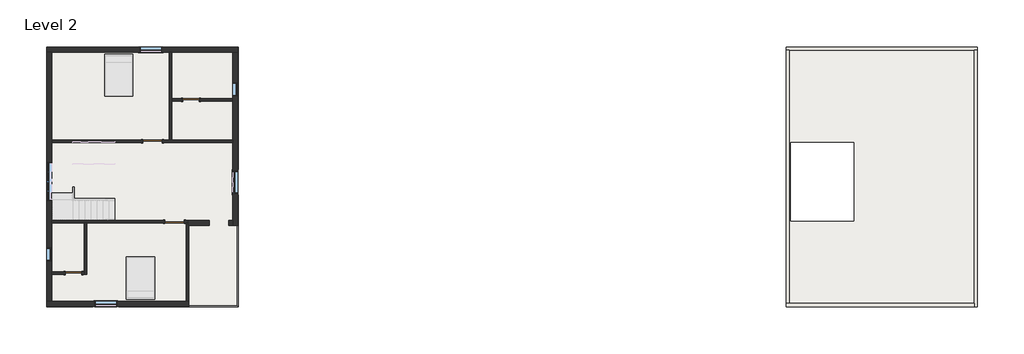
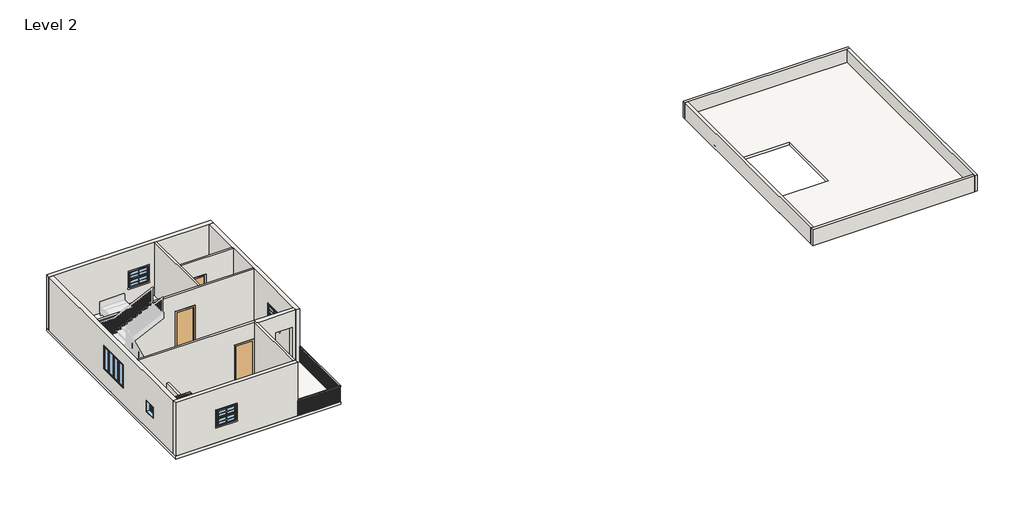
# One storey, part 1 of 3: 16 walls, 6 windows, 4 doors, 1 railing, 1 roof, 1 slab.
"""IFC4 building model written with IfcOpenShell, lengths in millimetres."""

from ifc_helpers import new_model, si_unit, frame, origin, place, context, project, spatial, polyline, outline, extrude, faceted_brep, transform, mapped, element, save
from components import door_f2b275c1, door_d8f5dbb5, single_flush_door_3_17d80c48, single_flush_door_3_5e62189b, window_fa0038f5, window_5487fb6d, window_f2d8fef0

model = new_model("IFC4")

# Units and contexts
model_context = context("Model", 3, world=origin())
ifc_project = project(units=[si_unit("LENGTHUNIT", "METRE", prefix="MILLI")], contexts=[model_context])

# Site, building, storey
site = spatial("IfcSite", under=ifc_project)
building = spatial("IfcBuilding", under=site)
storey = spatial("IfcBuildingStorey", under=building, Name="Level 2", Elevation=3048.0)

# Doors
placement = place(None, origin())
door_shape = door_f2b275c1(model_context)
element("IfcDoor", 1, ObjectType="Single-Flush : door 2'6\"", at=placement, inside=storey, context=model_context, shape_type="MappedRepresentation", body=[
    mapped(door_shape, transform((-16207.5289184, 4539.4100713, 3048.0), x_axis=(-1.0, 0.0, 0.0), y_axis=(0.0, -1.0, 0.0), z_axis=(0.0, 0.0, 1.0))),
])
door_2_shape = door_d8f5dbb5(model_context)
element("IfcDoor", 2, ObjectType="Single-Flush : door 2'6\"", at=placement, inside=storey, context=model_context, shape_type="MappedRepresentation", body=[
    mapped(door_2_shape, transform((-21693.9289184, -3575.8899287, 3048.0), x_axis=(1.0, 0.0, 0.0), y_axis=(0.0, 1.0, 0.0), z_axis=(0.0, 0.0, 1.0))),
])
single_flush_door_3_shape = single_flush_door_3_17d80c48(model_context)
element("IfcDoor", 3, ObjectType="Single-Flush : door 3'", at=placement, inside=storey, context=model_context, shape_type="MappedRepresentation", body=[
    mapped(single_flush_door_3_shape, transform((-18010.9289184, 2596.3100713, 3048.0), x_axis=(1.0, 0.0, 0.0), y_axis=(0.0, 1.0, 0.0), z_axis=(0.0, 0.0, 1.0))),
])
single_flush_door_3_2_shape = single_flush_door_3_5e62189b(model_context)
element("IfcDoor", 4, ObjectType="Single-Flush : door 3'", at=placement, inside=storey, context=model_context, shape_type="MappedRepresentation", body=[
    mapped(single_flush_door_3_2_shape, transform((-16982.2289184, -1175.5899287, 3048.0), x_axis=(1.0, 0.0, 0.0), y_axis=(0.0, 1.0, 0.0), z_axis=(0.0, 0.0, 1.0))),
])

# Railing
element("IfcRailing", 5, ObjectType="Handrail - Rectangular", at=placement, inside=storey, context=model_context, shape_type="SolidModel", body=[
    faceted_brep([(-16315.4789184, -5093.5399287, 3962.4), (-16315.4789184, -5093.5399287, 3911.6), (-16315.4789184, -5144.3399287, 3911.6), (-16315.4789184, -5144.3399287, 3962.4), (-14054.8789184, -5093.5399287, 3962.4), (-14054.8789184, -5093.5399287, 3911.6), (-14004.0789184, -5144.3399287, 3911.6), (-14004.0789184, -5144.3399287, 3962.4), (-14054.8789184, -1347.0399287, 3962.4), (-14004.0789184, -1347.0399287, 3962.4), (-14004.0789184, -1347.0399287, 3911.6), (-14054.8789184, -1347.0399287, 3911.6)], [[[0, 1, 2, 3]], [[1, 0, 4, 5]], [[2, 1, 5, 6]], [[3, 2, 6, 7]], [[0, 3, 7, 4]], [[8, 9, 10, 11]], [[5, 4, 8, 11]], [[6, 5, 11, 10]], [[7, 6, 10, 9]], [[4, 7, 9, 8]]]),
    extrude(outline(polyline([(-14019.9539184, -1369.2649287), (-14039.0039184, -1369.2649287), (-14039.0039184, -1350.2149287), (-14019.9539184, -1350.2149287), (-14019.9539184, -1369.2649287)])), frame((0.0, 0.0, 3048.0), z_axis=(0.0, 0.0, 1.0), x_axis=(1.0, 0.0, 0.0)), (0.0, 0.0, 1.0), 863.6),
    extrude(outline(polyline([(-14019.9539184, -1470.8649287), (-14039.0039184, -1470.8649287), (-14039.0039184, -1451.8149287), (-14019.9539184, -1451.8149287), (-14019.9539184, -1470.8649287)])), frame((0.0, 0.0, 3048.0), z_axis=(0.0, 0.0, 1.0), x_axis=(1.0, 0.0, 0.0)), (0.0, 0.0, 1.0), 863.6),
    extrude(outline(polyline([(-14019.9539184, -1572.4649287), (-14039.0039184, -1572.4649287), (-14039.0039184, -1553.4149287), (-14019.9539184, -1553.4149287), (-14019.9539184, -1572.4649287)])), frame((0.0, 0.0, 3048.0), z_axis=(0.0, 0.0, 1.0), x_axis=(1.0, 0.0, 0.0)), (0.0, 0.0, 1.0), 863.6),
    extrude(outline(polyline([(-14019.9539184, -1674.0649287), (-14039.0039184, -1674.0649287), (-14039.0039184, -1655.0149287), (-14019.9539184, -1655.0149287), (-14019.9539184, -1674.0649287)])), frame((0.0, 0.0, 3048.0), z_axis=(0.0, 0.0, 1.0), x_axis=(1.0, 0.0, 0.0)), (0.0, 0.0, 1.0), 863.6),
    extrude(outline(polyline([(-14019.9539184, -1775.6649287), (-14039.0039184, -1775.6649287), (-14039.0039184, -1756.6149287), (-14019.9539184, -1756.6149287), (-14019.9539184, -1775.6649287)])), frame((0.0, 0.0, 3048.0), z_axis=(0.0, 0.0, 1.0), x_axis=(1.0, 0.0, 0.0)), (0.0, 0.0, 1.0), 863.6),
    extrude(outline(polyline([(-14019.9539184, -1877.2649287), (-14039.0039184, -1877.2649287), (-14039.0039184, -1858.2149287), (-14019.9539184, -1858.2149287), (-14019.9539184, -1877.2649287)])), frame((0.0, 0.0, 3048.0), z_axis=(0.0, 0.0, 1.0), x_axis=(1.0, 0.0, 0.0)), (0.0, 0.0, 1.0), 863.6),
    extrude(outline(polyline([(-14019.9539184, -1978.8649287), (-14039.0039184, -1978.8649287), (-14039.0039184, -1959.8149287), (-14019.9539184, -1959.8149287), (-14019.9539184, -1978.8649287)])), frame((0.0, 0.0, 3048.0), z_axis=(0.0, 0.0, 1.0), x_axis=(1.0, 0.0, 0.0)), (0.0, 0.0, 1.0), 863.6),
    extrude(outline(polyline([(-14019.9539184, -2080.4649287), (-14039.0039184, -2080.4649287), (-14039.0039184, -2061.4149287), (-14019.9539184, -2061.4149287), (-14019.9539184, -2080.4649287)])), frame((0.0, 0.0, 3048.0), z_axis=(0.0, 0.0, 1.0), x_axis=(1.0, 0.0, 0.0)), (0.0, 0.0, 1.0), 863.6),
    extrude(outline(polyline([(-14019.9539184, -2182.0649287), (-14039.0039184, -2182.0649287), (-14039.0039184, -2163.0149287), (-14019.9539184, -2163.0149287), (-14019.9539184, -2182.0649287)])), frame((0.0, 0.0, 3048.0), z_axis=(0.0, 0.0, 1.0), x_axis=(1.0, 0.0, 0.0)), (0.0, 0.0, 1.0), 863.6),
    extrude(outline(polyline([(-14019.9539184, -2283.6649287), (-14039.0039184, -2283.6649287), (-14039.0039184, -2264.6149287), (-14019.9539184, -2264.6149287), (-14019.9539184, -2283.6649287)])), frame((0.0, 0.0, 3048.0), z_axis=(0.0, 0.0, 1.0), x_axis=(1.0, 0.0, 0.0)), (0.0, 0.0, 1.0), 863.6),
    extrude(outline(polyline([(-14019.9539184, -2385.2649287), (-14039.0039184, -2385.2649287), (-14039.0039184, -2366.2149287), (-14019.9539184, -2366.2149287), (-14019.9539184, -2385.2649287)])), frame((0.0, 0.0, 3048.0), z_axis=(0.0, 0.0, 1.0), x_axis=(1.0, 0.0, 0.0)), (0.0, 0.0, 1.0), 863.6),
    extrude(outline(polyline([(-14019.9539184, -2486.8649287), (-14039.0039184, -2486.8649287), (-14039.0039184, -2467.8149287), (-14019.9539184, -2467.8149287), (-14019.9539184, -2486.8649287)])), frame((0.0, 0.0, 3048.0), z_axis=(0.0, 0.0, 1.0), x_axis=(1.0, 0.0, 0.0)), (0.0, 0.0, 1.0), 863.6),
    extrude(outline(polyline([(-14019.9539184, -2588.4649287), (-14039.0039184, -2588.4649287), (-14039.0039184, -2569.4149287), (-14019.9539184, -2569.4149287), (-14019.9539184, -2588.4649287)])), frame((0.0, 0.0, 3048.0), z_axis=(0.0, 0.0, 1.0), x_axis=(1.0, 0.0, 0.0)), (0.0, 0.0, 1.0), 863.6),
    extrude(outline(polyline([(-14019.9539184, -2690.0649287), (-14039.0039184, -2690.0649287), (-14039.0039184, -2671.0149287), (-14019.9539184, -2671.0149287), (-14019.9539184, -2690.0649287)])), frame((0.0, 0.0, 3048.0), z_axis=(0.0, 0.0, 1.0), x_axis=(1.0, 0.0, 0.0)), (0.0, 0.0, 1.0), 863.6),
    extrude(outline(polyline([(-14019.9539184, -2791.6649287), (-14039.0039184, -2791.6649287), (-14039.0039184, -2772.6149287), (-14019.9539184, -2772.6149287), (-14019.9539184, -2791.6649287)])), frame((0.0, 0.0, 3048.0), z_axis=(0.0, 0.0, 1.0), x_axis=(1.0, 0.0, 0.0)), (0.0, 0.0, 1.0), 863.6),
    extrude(outline(polyline([(-14019.9539184, -2893.2649287), (-14039.0039184, -2893.2649287), (-14039.0039184, -2874.2149287), (-14019.9539184, -2874.2149287), (-14019.9539184, -2893.2649287)])), frame((0.0, 0.0, 3048.0), z_axis=(0.0, 0.0, 1.0), x_axis=(1.0, 0.0, 0.0)), (0.0, 0.0, 1.0), 863.6),
    extrude(outline(polyline([(-14019.9539184, -2994.8649287), (-14039.0039184, -2994.8649287), (-14039.0039184, -2975.8149287), (-14019.9539184, -2975.8149287), (-14019.9539184, -2994.8649287)])), frame((0.0, 0.0, 3048.0), z_axis=(0.0, 0.0, 1.0), x_axis=(1.0, 0.0, 0.0)), (0.0, 0.0, 1.0), 863.6),
    extrude(outline(polyline([(-14019.9539184, -3096.4649287), (-14039.0039184, -3096.4649287), (-14039.0039184, -3077.4149287), (-14019.9539184, -3077.4149287), (-14019.9539184, -3096.4649287)])), frame((0.0, 0.0, 3048.0), z_axis=(0.0, 0.0, 1.0), x_axis=(1.0, 0.0, 0.0)), (0.0, 0.0, 1.0), 863.6),
    extrude(outline(polyline([(-14019.9539184, -3198.0649287), (-14039.0039184, -3198.0649287), (-14039.0039184, -3179.0149287), (-14019.9539184, -3179.0149287), (-14019.9539184, -3198.0649287)])), frame((0.0, 0.0, 3048.0), z_axis=(0.0, 0.0, 1.0), x_axis=(1.0, 0.0, 0.0)), (0.0, 0.0, 1.0), 863.6),
    extrude(outline(polyline([(-14019.9539184, -3299.6649287), (-14039.0039184, -3299.6649287), (-14039.0039184, -3280.6149287), (-14019.9539184, -3280.6149287), (-14019.9539184, -3299.6649287)])), frame((0.0, 0.0, 3048.0), z_axis=(0.0, 0.0, 1.0), x_axis=(1.0, 0.0, 0.0)), (0.0, 0.0, 1.0), 863.6),
    extrude(outline(polyline([(-14019.9539184, -3401.2649287), (-14039.0039184, -3401.2649287), (-14039.0039184, -3382.2149287), (-14019.9539184, -3382.2149287), (-14019.9539184, -3401.2649287)])), frame((0.0, 0.0, 3048.0), z_axis=(0.0, 0.0, 1.0), x_axis=(1.0, 0.0, 0.0)), (0.0, 0.0, 1.0), 863.6),
    extrude(outline(polyline([(-14019.9539184, -3502.8649287), (-14039.0039184, -3502.8649287), (-14039.0039184, -3483.8149287), (-14019.9539184, -3483.8149287), (-14019.9539184, -3502.8649287)])), frame((0.0, 0.0, 3048.0), z_axis=(0.0, 0.0, 1.0), x_axis=(1.0, 0.0, 0.0)), (0.0, 0.0, 1.0), 863.6),
    extrude(outline(polyline([(-14019.9539184, -3604.4649287), (-14039.0039184, -3604.4649287), (-14039.0039184, -3585.4149287), (-14019.9539184, -3585.4149287), (-14019.9539184, -3604.4649287)])), frame((0.0, 0.0, 3048.0), z_axis=(0.0, 0.0, 1.0), x_axis=(1.0, 0.0, 0.0)), (0.0, 0.0, 1.0), 863.6),
    extrude(outline(polyline([(-14019.9539184, -3706.0649287), (-14039.0039184, -3706.0649287), (-14039.0039184, -3687.0149287), (-14019.9539184, -3687.0149287), (-14019.9539184, -3706.0649287)])), frame((0.0, 0.0, 3048.0), z_axis=(0.0, 0.0, 1.0), x_axis=(1.0, 0.0, 0.0)), (0.0, 0.0, 1.0), 863.6),
    extrude(outline(polyline([(-14019.9539184, -3807.6649287), (-14039.0039184, -3807.6649287), (-14039.0039184, -3788.6149287), (-14019.9539184, -3788.6149287), (-14019.9539184, -3807.6649287)])), frame((0.0, 0.0, 3048.0), z_axis=(0.0, 0.0, 1.0), x_axis=(1.0, 0.0, 0.0)), (0.0, 0.0, 1.0), 863.6),
    extrude(outline(polyline([(-14019.9539184, -3909.2649287), (-14039.0039184, -3909.2649287), (-14039.0039184, -3890.2149287), (-14019.9539184, -3890.2149287), (-14019.9539184, -3909.2649287)])), frame((0.0, 0.0, 3048.0), z_axis=(0.0, 0.0, 1.0), x_axis=(1.0, 0.0, 0.0)), (0.0, 0.0, 1.0), 863.6),
    extrude(outline(polyline([(-14019.9539184, -4010.8649287), (-14039.0039184, -4010.8649287), (-14039.0039184, -3991.8149287), (-14019.9539184, -3991.8149287), (-14019.9539184, -4010.8649287)])), frame((0.0, 0.0, 3048.0), z_axis=(0.0, 0.0, 1.0), x_axis=(1.0, 0.0, 0.0)), (0.0, 0.0, 1.0), 863.6),
    extrude(outline(polyline([(-14019.9539184, -4112.4649287), (-14039.0039184, -4112.4649287), (-14039.0039184, -4093.4149287), (-14019.9539184, -4093.4149287), (-14019.9539184, -4112.4649287)])), frame((0.0, 0.0, 3048.0), z_axis=(0.0, 0.0, 1.0), x_axis=(1.0, 0.0, 0.0)), (0.0, 0.0, 1.0), 863.6),
    extrude(outline(polyline([(-14019.9539184, -4214.0649287), (-14039.0039184, -4214.0649287), (-14039.0039184, -4195.0149287), (-14019.9539184, -4195.0149287), (-14019.9539184, -4214.0649287)])), frame((0.0, 0.0, 3048.0), z_axis=(0.0, 0.0, 1.0), x_axis=(1.0, 0.0, 0.0)), (0.0, 0.0, 1.0), 863.6),
    extrude(outline(polyline([(-14019.9539184, -4315.6649287), (-14039.0039184, -4315.6649287), (-14039.0039184, -4296.6149287), (-14019.9539184, -4296.6149287), (-14019.9539184, -4315.6649287)])), frame((0.0, 0.0, 3048.0), z_axis=(0.0, 0.0, 1.0), x_axis=(1.0, 0.0, 0.0)), (0.0, 0.0, 1.0), 863.6),
    extrude(outline(polyline([(-14019.9539184, -4417.2649287), (-14039.0039184, -4417.2649287), (-14039.0039184, -4398.2149287), (-14019.9539184, -4398.2149287), (-14019.9539184, -4417.2649287)])), frame((0.0, 0.0, 3048.0), z_axis=(0.0, 0.0, 1.0), x_axis=(1.0, 0.0, 0.0)), (0.0, 0.0, 1.0), 863.6),
    extrude(outline(polyline([(-14019.9539184, -4518.8649287), (-14039.0039184, -4518.8649287), (-14039.0039184, -4499.8149287), (-14019.9539184, -4499.8149287), (-14019.9539184, -4518.8649287)])), frame((0.0, 0.0, 3048.0), z_axis=(0.0, 0.0, 1.0), x_axis=(1.0, 0.0, 0.0)), (0.0, 0.0, 1.0), 863.6),
    extrude(outline(polyline([(-14019.9539184, -4620.4649287), (-14039.0039184, -4620.4649287), (-14039.0039184, -4601.4149287), (-14019.9539184, -4601.4149287), (-14019.9539184, -4620.4649287)])), frame((0.0, 0.0, 3048.0), z_axis=(0.0, 0.0, 1.0), x_axis=(1.0, 0.0, 0.0)), (0.0, 0.0, 1.0), 863.6),
    extrude(outline(polyline([(-14019.9539184, -4722.0649287), (-14039.0039184, -4722.0649287), (-14039.0039184, -4703.0149287), (-14019.9539184, -4703.0149287), (-14019.9539184, -4722.0649287)])), frame((0.0, 0.0, 3048.0), z_axis=(0.0, 0.0, 1.0), x_axis=(1.0, 0.0, 0.0)), (0.0, 0.0, 1.0), 863.6),
    extrude(outline(polyline([(-14019.9539184, -4823.6649287), (-14039.0039184, -4823.6649287), (-14039.0039184, -4804.6149287), (-14019.9539184, -4804.6149287), (-14019.9539184, -4823.6649287)])), frame((0.0, 0.0, 3048.0), z_axis=(0.0, 0.0, 1.0), x_axis=(1.0, 0.0, 0.0)), (0.0, 0.0, 1.0), 863.6),
    extrude(outline(polyline([(-14019.9539184, -4925.2649287), (-14039.0039184, -4925.2649287), (-14039.0039184, -4906.2149287), (-14019.9539184, -4906.2149287), (-14019.9539184, -4925.2649287)])), frame((0.0, 0.0, 3048.0), z_axis=(0.0, 0.0, 1.0), x_axis=(1.0, 0.0, 0.0)), (0.0, 0.0, 1.0), 863.6),
    extrude(outline(polyline([(-14019.9539184, -5026.8649287), (-14039.0039184, -5026.8649287), (-14039.0039184, -5007.8149287), (-14019.9539184, -5007.8149287), (-14019.9539184, -5026.8649287)])), frame((0.0, 0.0, 3048.0), z_axis=(0.0, 0.0, 1.0), x_axis=(1.0, 0.0, 0.0)), (0.0, 0.0, 1.0), 863.6),
    extrude(outline(polyline([(-14089.8039184, -5128.4649287), (-14089.8039184, -5109.4149287), (-14070.7539184, -5109.4149287), (-14070.7539184, -5128.4649287), (-14089.8039184, -5128.4649287)])), frame((0.0, 0.0, 3048.0), z_axis=(0.0, 0.0, 1.0), x_axis=(1.0, 0.0, 0.0)), (0.0, 0.0, 1.0), 863.6),
    extrude(outline(polyline([(-14191.4039184, -5128.4649287), (-14191.4039184, -5109.4149287), (-14172.3539184, -5109.4149287), (-14172.3539184, -5128.4649287), (-14191.4039184, -5128.4649287)])), frame((0.0, 0.0, 3048.0), z_axis=(0.0, 0.0, 1.0), x_axis=(1.0, 0.0, 0.0)), (0.0, 0.0, 1.0), 863.6),
    extrude(outline(polyline([(-14293.0039184, -5128.4649287), (-14293.0039184, -5109.4149287), (-14273.9539184, -5109.4149287), (-14273.9539184, -5128.4649287), (-14293.0039184, -5128.4649287)])), frame((0.0, 0.0, 3048.0), z_axis=(0.0, 0.0, 1.0), x_axis=(1.0, 0.0, 0.0)), (0.0, 0.0, 1.0), 863.6),
    extrude(outline(polyline([(-14394.6039184, -5128.4649287), (-14394.6039184, -5109.4149287), (-14375.5539184, -5109.4149287), (-14375.5539184, -5128.4649287), (-14394.6039184, -5128.4649287)])), frame((0.0, 0.0, 3048.0), z_axis=(0.0, 0.0, 1.0), x_axis=(1.0, 0.0, 0.0)), (0.0, 0.0, 1.0), 863.6),
    extrude(outline(polyline([(-14496.2039184, -5128.4649287), (-14496.2039184, -5109.4149287), (-14477.1539184, -5109.4149287), (-14477.1539184, -5128.4649287), (-14496.2039184, -5128.4649287)])), frame((0.0, 0.0, 3048.0), z_axis=(0.0, 0.0, 1.0), x_axis=(1.0, 0.0, 0.0)), (0.0, 0.0, 1.0), 863.6),
    extrude(outline(polyline([(-14597.8039184, -5128.4649287), (-14597.8039184, -5109.4149287), (-14578.7539184, -5109.4149287), (-14578.7539184, -5128.4649287), (-14597.8039184, -5128.4649287)])), frame((0.0, 0.0, 3048.0), z_axis=(0.0, 0.0, 1.0), x_axis=(1.0, 0.0, 0.0)), (0.0, 0.0, 1.0), 863.6),
    extrude(outline(polyline([(-14699.4039184, -5128.4649287), (-14699.4039184, -5109.4149287), (-14680.3539184, -5109.4149287), (-14680.3539184, -5128.4649287), (-14699.4039184, -5128.4649287)])), frame((0.0, 0.0, 3048.0), z_axis=(0.0, 0.0, 1.0), x_axis=(1.0, 0.0, 0.0)), (0.0, 0.0, 1.0), 863.6),
    extrude(outline(polyline([(-14801.0039184, -5128.4649287), (-14801.0039184, -5109.4149287), (-14781.9539184, -5109.4149287), (-14781.9539184, -5128.4649287), (-14801.0039184, -5128.4649287)])), frame((0.0, 0.0, 3048.0), z_axis=(0.0, 0.0, 1.0), x_axis=(1.0, 0.0, 0.0)), (0.0, 0.0, 1.0), 863.6),
    extrude(outline(polyline([(-14902.6039184, -5128.4649287), (-14902.6039184, -5109.4149287), (-14883.5539184, -5109.4149287), (-14883.5539184, -5128.4649287), (-14902.6039184, -5128.4649287)])), frame((0.0, 0.0, 3048.0), z_axis=(0.0, 0.0, 1.0), x_axis=(1.0, 0.0, 0.0)), (0.0, 0.0, 1.0), 863.6),
    extrude(outline(polyline([(-15004.2039184, -5128.4649287), (-15004.2039184, -5109.4149287), (-14985.1539184, -5109.4149287), (-14985.1539184, -5128.4649287), (-15004.2039184, -5128.4649287)])), frame((0.0, 0.0, 3048.0), z_axis=(0.0, 0.0, 1.0), x_axis=(1.0, 0.0, 0.0)), (0.0, 0.0, 1.0), 863.6),
    extrude(outline(polyline([(-15105.8039184, -5128.4649287), (-15105.8039184, -5109.4149287), (-15086.7539184, -5109.4149287), (-15086.7539184, -5128.4649287), (-15105.8039184, -5128.4649287)])), frame((0.0, 0.0, 3048.0), z_axis=(0.0, 0.0, 1.0), x_axis=(1.0, 0.0, 0.0)), (0.0, 0.0, 1.0), 863.6),
    extrude(outline(polyline([(-15207.4039184, -5128.4649287), (-15207.4039184, -5109.4149287), (-15188.3539184, -5109.4149287), (-15188.3539184, -5128.4649287), (-15207.4039184, -5128.4649287)])), frame((0.0, 0.0, 3048.0), z_axis=(0.0, 0.0, 1.0), x_axis=(1.0, 0.0, 0.0)), (0.0, 0.0, 1.0), 863.6),
    extrude(outline(polyline([(-15309.0039184, -5128.4649287), (-15309.0039184, -5109.4149287), (-15289.9539184, -5109.4149287), (-15289.9539184, -5128.4649287), (-15309.0039184, -5128.4649287)])), frame((0.0, 0.0, 3048.0), z_axis=(0.0, 0.0, 1.0), x_axis=(1.0, 0.0, 0.0)), (0.0, 0.0, 1.0), 863.6),
    extrude(outline(polyline([(-15410.6039184, -5128.4649287), (-15410.6039184, -5109.4149287), (-15391.5539184, -5109.4149287), (-15391.5539184, -5128.4649287), (-15410.6039184, -5128.4649287)])), frame((0.0, 0.0, 3048.0), z_axis=(0.0, 0.0, 1.0), x_axis=(1.0, 0.0, 0.0)), (0.0, 0.0, 1.0), 863.6),
    extrude(outline(polyline([(-15512.2039184, -5128.4649287), (-15512.2039184, -5109.4149287), (-15493.1539184, -5109.4149287), (-15493.1539184, -5128.4649287), (-15512.2039184, -5128.4649287)])), frame((0.0, 0.0, 3048.0), z_axis=(0.0, 0.0, 1.0), x_axis=(1.0, 0.0, 0.0)), (0.0, 0.0, 1.0), 863.6),
    extrude(outline(polyline([(-15613.8039184, -5128.4649287), (-15613.8039184, -5109.4149287), (-15594.7539184, -5109.4149287), (-15594.7539184, -5128.4649287), (-15613.8039184, -5128.4649287)])), frame((0.0, 0.0, 3048.0), z_axis=(0.0, 0.0, 1.0), x_axis=(1.0, 0.0, 0.0)), (0.0, 0.0, 1.0), 863.6),
    extrude(outline(polyline([(-15715.4039184, -5128.4649287), (-15715.4039184, -5109.4149287), (-15696.3539184, -5109.4149287), (-15696.3539184, -5128.4649287), (-15715.4039184, -5128.4649287)])), frame((0.0, 0.0, 3048.0), z_axis=(0.0, 0.0, 1.0), x_axis=(1.0, 0.0, 0.0)), (0.0, 0.0, 1.0), 863.6),
    extrude(outline(polyline([(-15817.0039184, -5128.4649287), (-15817.0039184, -5109.4149287), (-15797.9539184, -5109.4149287), (-15797.9539184, -5128.4649287), (-15817.0039184, -5128.4649287)])), frame((0.0, 0.0, 3048.0), z_axis=(0.0, 0.0, 1.0), x_axis=(1.0, 0.0, 0.0)), (0.0, 0.0, 1.0), 863.6),
    extrude(outline(polyline([(-15918.6039184, -5128.4649287), (-15918.6039184, -5109.4149287), (-15899.5539184, -5109.4149287), (-15899.5539184, -5128.4649287), (-15918.6039184, -5128.4649287)])), frame((0.0, 0.0, 3048.0), z_axis=(0.0, 0.0, 1.0), x_axis=(1.0, 0.0, 0.0)), (0.0, 0.0, 1.0), 863.6),
    extrude(outline(polyline([(-16020.2039184, -5128.4649287), (-16020.2039184, -5109.4149287), (-16001.1539184, -5109.4149287), (-16001.1539184, -5128.4649287), (-16020.2039184, -5128.4649287)])), frame((0.0, 0.0, 3048.0), z_axis=(0.0, 0.0, 1.0), x_axis=(1.0, 0.0, 0.0)), (0.0, 0.0, 1.0), 863.6),
    extrude(outline(polyline([(-16121.8039184, -5128.4649287), (-16121.8039184, -5109.4149287), (-16102.7539184, -5109.4149287), (-16102.7539184, -5128.4649287), (-16121.8039184, -5128.4649287)])), frame((0.0, 0.0, 3048.0), z_axis=(0.0, 0.0, 1.0), x_axis=(1.0, 0.0, 0.0)), (0.0, 0.0, 1.0), 863.6),
    extrude(outline(polyline([(-16223.4039184, -5128.4649287), (-16223.4039184, -5109.4149287), (-16204.3539184, -5109.4149287), (-16204.3539184, -5128.4649287), (-16223.4039184, -5128.4649287)])), frame((0.0, 0.0, 3048.0), z_axis=(0.0, 0.0, 1.0), x_axis=(1.0, 0.0, 0.0)), (0.0, 0.0, 1.0), 863.6),
    extrude(outline(polyline([(-14039.0039184, -5128.4649287), (-14039.0039184, -5109.4149287), (-14019.9539184, -5109.4149287), (-14019.9539184, -5128.4649287), (-14039.0039184, -5128.4649287)])), frame((0.0, 0.0, 3048.0), z_axis=(0.0, 0.0, 1.0), x_axis=(1.0, 0.0, 0.0)), (0.0, 0.0, 1.0), 863.6),
    extrude(outline(polyline([(-14019.9539184, -1366.0899287), (-14039.0039184, -1366.0899287), (-14039.0039184, -1347.0399287), (-14019.9539184, -1347.0399287), (-14019.9539184, -1366.0899287)])), frame((0.0, 0.0, 3048.0), z_axis=(0.0, 0.0, 1.0), x_axis=(1.0, 0.0, 0.0)), (0.0, 0.0, 1.0), 863.6),
    extrude(outline(polyline([(-16315.4789184, -5128.4649287), (-16315.4789184, -5109.4149287), (-16296.4289184, -5109.4149287), (-16296.4289184, -5128.4649287), (-16315.4789184, -5128.4649287)])), frame((0.0, 0.0, 3048.0), z_axis=(0.0, 0.0, 1.0), x_axis=(1.0, 0.0, 0.0)), (0.0, 0.0, 1.0), 863.6),
])

# Roof
element("IfcRoof", 6, ObjectType="Generic - 12\"", at=placement, inside=storey, context=model_context, shape_type="SweptSolid", body=[
    extrude(outline(polyline([(11575.242447, -5144.3399287), (11575.242447, 6996.8600713), (20516.042447, 6996.8600713), (20516.042447, -5144.3399287), (11575.242447, -5144.3399287)]), holes=[polyline([(11803.842447, 2539.1600713), (11803.842447, -1118.4399287), (14750.242447, -1118.4399287), (14750.242447, 2539.1600713), (11803.842447, 2539.1600713)])]), frame((0.0, 0.0, 3048.0), z_axis=(0.0, 0.0, 1.0), x_axis=(1.0, 0.0, 0.0)), (0.0, 0.0, 1.0), 152.4),
])

# Slab
element("IfcSlab", 7, ObjectType="floor 6\"", at=placement, inside=storey, context=model_context, shape_type="SweptSolid", body=[
    extrude(outline(polyline([(-14004.0789184, 6996.8600713), (-14004.0789184, -5144.3399287), (-22944.8789184, -5144.3399287), (-22944.8789184, 6996.8600713), (-14004.0789184, 6996.8600713)])), frame((0.0, 0.0, 2895.6), z_axis=(0.0, 0.0, 1.0), x_axis=(1.0, 0.0, 0.0)), (0.0, 0.0, 1.0), 152.4),
])

# Walls
element("IfcWall", 8, ObjectType="WALL 4.5\"", at=placement, inside=storey, context=model_context, shape_type="Brep", body=[
    faceted_brep([(-16372.6289184, -1118.4399287, 3048.0), (-16525.0289184, -1118.4399287, 3048.0), (-16525.0289184, -1118.4399287, 5080.0), (-17439.4289184, -1118.4399287, 5080.0), (-17439.4289184, -1118.4399287, 3048.0), (-22716.2789184, -1118.4399287, 3048.0), (-22716.2789184, -1118.4399287, 6096.0), (-16372.6289184, -1118.4399287, 6096.0), (-16525.0289184, -1232.7399287, 5080.0), (-16525.0289184, -1232.7399287, 3048.0), (-16429.7789184, -1232.7399287, 3048.0), (-16372.6289184, -1232.7399287, 3048.0), (-16372.6289184, -1232.7399287, 6096.0), (-16429.7789184, -1232.7399287, 6096.0), (-22716.2789184, -1232.7399287, 6096.0), (-22716.2789184, -1232.7399287, 3048.0), (-21192.2789184, -1232.7399287, 3048.0), (-21077.9789184, -1232.7399287, 3048.0), (-17439.4289184, -1232.7399287, 3048.0), (-17439.4289184, -1232.7399287, 5080.0)], [[[0, 1, 2, 3, 4, 5, 6, 7]], [[8, 9, 10, 11, 12, 13, 14, 15, 16, 17, 18, 19]], [[11, 10, 9, 1, 0]], [[18, 17, 16, 15, 5, 4]], [[7, 6, 14, 13, 12]], [[0, 7, 12, 11]], [[6, 5, 15, 14]], [[2, 1, 9, 8]], [[3, 2, 8, 19]], [[4, 3, 19, 18]]]),
])
element("IfcWall", 9, ObjectType="WALL 4.5\"", at=placement, inside=storey, context=model_context, shape_type="Brep", body=[
    faceted_brep([(-14258.0789184, 2653.4600713, 3048.0), (-17115.5789184, 2653.4600713, 3048.0), (-17229.8789184, 2653.4600713, 3048.0), (-17553.7289184, 2653.4600713, 3048.0), (-17553.7289184, 2653.4600713, 5080.0), (-18468.1289184, 2653.4600713, 5080.0), (-18468.1289184, 2653.4600713, 3048.0), (-22716.2789184, 2653.4600713, 3048.0), (-22716.2789184, 2653.4600713, 6096.0), (-17229.8789184, 2653.4600713, 6096.0), (-17115.5789184, 2653.4600713, 6096.0), (-14258.0789184, 2653.4600713, 6096.0), (-17553.7289184, 2539.1600713, 5080.0), (-17553.7289184, 2539.1600713, 3048.0), (-14258.0789184, 2539.1600713, 3048.0), (-14258.0789184, 2539.1600713, 6096.0), (-22716.2789184, 2539.1600713, 6096.0), (-22716.2789184, 2539.1600713, 3048.0), (-18468.1289184, 2539.1600713, 3048.0), (-18468.1289184, 2539.1600713, 5080.0)], [[[0, 1, 2, 3, 4, 5, 6, 7, 8, 9, 10, 11]], [[12, 13, 14, 15, 16, 17, 18, 19]], [[18, 17, 7, 6]], [[14, 13, 3, 2, 1, 0]], [[11, 10, 9, 8, 16, 15]], [[0, 11, 15, 14]], [[8, 7, 17, 16]], [[4, 3, 13, 12]], [[5, 4, 12, 19]], [[6, 5, 19, 18]]]),
])
element("IfcWall", 10, ObjectType="WALL 4.5\"", at=placement, inside=storey, context=model_context, shape_type="Brep", body=[
    faceted_brep([(-17229.8789184, 6768.2600713, 3048.0), (-17229.8789184, 2653.4600713, 3048.0), (-17229.8789184, 2653.4600713, 6096.0), (-17229.8789184, 6768.2600713, 6096.0), (-17115.5789184, 6768.2600713, 3048.0), (-17115.5789184, 6768.2600713, 6096.0), (-17115.5789184, 4596.5600713, 6096.0), (-17115.5789184, 4482.2600713, 6096.0), (-17115.5789184, 2653.4600713, 6096.0), (-17115.5789184, 2653.4600713, 3048.0), (-17115.5789184, 4482.2600713, 3048.0), (-17115.5789184, 4596.5600713, 3048.0)], [[[0, 1, 2, 3]], [[4, 5, 6, 7, 8, 9, 10, 11]], [[1, 0, 4, 11, 10, 9]], [[3, 2, 8, 7, 6, 5]], [[0, 3, 5, 4]], [[2, 1, 9, 8]]]),
])
element("IfcWall", 11, ObjectType="WALL 4.5\"", at=placement, inside=storey, context=model_context, shape_type="SweptSolid", body=[
    extrude(outline(polyline([(3048.0, -17115.5789184), (3048.0, -16588.5289184), (5080.0, -16588.5289184), (5080.0, -15826.5289184), (3048.0, -15826.5289184), (3048.0, -14258.0789184), (6096.0, -14258.0789184), (6096.0, -17115.5789184), (3048.0, -17115.5789184)])), frame((0.0, 4482.2600713, 0.0), z_axis=(0.0, 1.0, 0.0), x_axis=(0.0, 0.0, 1.0)), (0.0, 0.0, 1.0), 114.3),
])
element("IfcWall", 12, ObjectType="WALL 4.5\"", at=placement, inside=storey, context=model_context, shape_type="SweptSolid", body=[
    extrude(outline(polyline([(-16315.4789184, -1347.0399287), (-16315.4789184, -4890.3399287), (-16429.7789184, -4890.3399287), (-16429.7789184, -1232.7399287), (-16372.6289184, -1232.7399287), (-16372.6289184, -1347.0399287), (-16315.4789184, -1347.0399287)])), frame((0.0, 0.0, 3048.0), z_axis=(0.0, 0.0, 1.0), x_axis=(1.0, 0.0, 0.0)), (0.0, 0.0, 1.0), 3048.0),
])
element("IfcWall", 13, ObjectType="WALL 4.5\"", at=placement, inside=storey, context=model_context, shape_type="Brep", body=[
    faceted_brep([(-21192.2789184, -1232.7399287, 3048.0), (-21192.2789184, -3518.7399287, 3048.0), (-21192.2789184, -3633.0399287, 3048.0), (-21192.2789184, -3633.0399287, 4267.2), (-21192.2789184, -3518.7399287, 4267.2), (-21192.2789184, -1232.7399287, 4267.2), (-21077.9789184, -1232.7399287, 3048.0), (-21077.9789184, -1232.7399287, 4267.2), (-21077.9789184, -3633.0399287, 4267.2), (-21077.9789184, -3633.0399287, 3048.0)], [[[0, 1, 2, 3, 4, 5]], [[6, 7, 8, 9]], [[2, 1, 0, 6, 9]], [[5, 4, 3, 8, 7]], [[0, 5, 7, 6]], [[3, 2, 9, 8]]]),
])
element("IfcWall", 14, ObjectType="WALL 4.5\"", at=placement, inside=storey, context=model_context, shape_type="SweptSolid", body=[
    extrude(outline(polyline([(-21192.2789184, -3518.7399287), (-21192.2789184, -3633.0399287), (-21312.9289184, -3633.0399287), (-21312.9289184, -3518.7399287), (-21192.2789184, -3518.7399287)])), frame((0.0, 0.0, 3048.0), z_axis=(0.0, 0.0, 1.0), x_axis=(1.0, 0.0, 0.0)), (0.0, 0.0, 1.0), 1219.2),
    extrude(outline(polyline([(-22716.2789184, -3633.0399287), (-22716.2789184, -3518.7399287), (-22074.9289184, -3518.7399287), (-22074.9289184, -3633.0399287), (-22716.2789184, -3633.0399287)])), frame((0.0, 0.0, 3048.0), z_axis=(0.0, 0.0, 1.0), x_axis=(1.0, 0.0, 0.0)), (0.0, 0.0, 1.0), 1219.2),
])
element("IfcWall", 15, ObjectType="WALL 9\"", at=placement, inside=storey, context=model_context, shape_type="Brep", body=[
    faceted_brep([(-22944.8789184, 6768.2600713, 3048.0), (-22716.2789184, 6768.2600713, 3048.0), (-17229.8789184, 6768.2600713, 3048.0), (-17115.5789184, 6768.2600713, 3048.0), (-14258.0789184, 6768.2600713, 3048.0), (-14029.4789184, 6768.2600713, 3048.0), (-14029.4789184, 6768.2600713, 6096.0), (-14258.0789184, 6768.2600713, 6096.0), (-17115.5789184, 6768.2600713, 6096.0), (-17229.8789184, 6768.2600713, 6096.0), (-22716.2789184, 6768.2600713, 6096.0), (-22944.8789184, 6768.2600713, 6096.0), (-18607.8289184, 6768.2600713, 4876.8), (-17566.4289184, 6768.2600713, 4876.8), (-17566.4289184, 6768.2600713, 3962.4), (-18607.8289184, 6768.2600713, 3962.4), (-22944.8789184, 6996.8600713, 3048.0), (-22944.8789184, 6996.8600713, 6096.0), (-14029.4789184, 6996.8600713, 6096.0), (-14029.4789184, 6996.8600713, 3048.0), (-18607.8289184, 6996.8600713, 4876.8), (-18607.8289184, 6996.8600713, 3962.4), (-17566.4289184, 6996.8600713, 3962.4), (-17566.4289184, 6996.8600713, 4876.8)], [[[0, 1, 2, 3, 4, 5, 6, 7, 8, 9, 10, 11], [12, 13, 14, 15]], [[16, 17, 18, 19], [20, 21, 22, 23]], [[5, 4, 3, 2, 1, 0, 16, 19]], [[11, 10, 9, 8, 7, 6, 18, 17]], [[6, 5, 19, 18]], [[0, 11, 17, 16]], [[21, 20, 12, 15]], [[22, 21, 15, 14]], [[23, 22, 14, 13]], [[20, 23, 13, 12]]]),
])
element("IfcWall", 16, ObjectType="WALL 9\"", at=placement, inside=storey, context=model_context, shape_type="Brep", body=[
    faceted_brep([(-14258.0789184, 6768.2600713, 3048.0), (-14258.0789184, 4596.5600713, 3048.0), (-14258.0789184, 4482.2600713, 3048.0), (-14258.0789184, 2653.4600713, 3048.0), (-14258.0789184, 2539.1600713, 3048.0), (-14258.0789184, -1118.4399287, 3048.0), (-14258.0789184, -1347.0399287, 3048.0), (-14258.0789184, -1347.0399287, 6096.0), (-14258.0789184, -1118.4399287, 6096.0), (-14258.0789184, 2539.1600713, 6096.0), (-14258.0789184, 2653.4600713, 6096.0), (-14258.0789184, 4482.2600713, 6096.0), (-14258.0789184, 4596.5600713, 6096.0), (-14258.0789184, 6768.2600713, 6096.0), (-14258.0789184, 1202.4850713, 4876.8), (-14258.0789184, 161.0850713, 4876.8), (-14258.0789184, 161.0850713, 3962.4), (-14258.0789184, 1202.4850713, 3962.4), (-14258.0789184, 5326.8100713, 4572.0), (-14258.0789184, 4717.2100713, 4572.0), (-14258.0789184, 4717.2100713, 3962.4), (-14258.0789184, 5326.8100713, 3962.4), (-14029.4789184, 6768.2600713, 3048.0), (-14029.4789184, 6768.2600713, 6096.0), (-14029.4789184, -1347.0399287, 6096.0), (-14029.4789184, -1347.0399287, 3048.0), (-14029.4789184, 1202.4850713, 4876.8), (-14029.4789184, 1202.4850713, 3962.4), (-14029.4789184, 161.0850713, 3962.4), (-14029.4789184, 161.0850713, 4876.8), (-14029.4789184, 5326.8100713, 4572.0), (-14029.4789184, 5326.8100713, 3962.4), (-14029.4789184, 4717.2100713, 3962.4), (-14029.4789184, 4717.2100713, 4572.0)], [[[0, 1, 2, 3, 4, 5, 6, 7, 8, 9, 10, 11, 12, 13], [14, 15, 16, 17], [18, 19, 20, 21]], [[22, 23, 24, 25], [26, 27, 28, 29], [30, 31, 32, 33]], [[6, 5, 4, 3, 2, 1, 0, 22, 25]], [[13, 12, 11, 10, 9, 8, 7, 24, 23]], [[0, 13, 23, 22]], [[7, 6, 25, 24]], [[27, 26, 14, 17]], [[28, 27, 17, 16]], [[29, 28, 16, 15]], [[26, 29, 15, 14]], [[31, 30, 18, 21]], [[32, 31, 21, 20]], [[33, 32, 20, 19]], [[30, 33, 19, 18]]]),
])
element("IfcWall", 17, ObjectType="WALL 9\"", at=placement, inside=storey, context=model_context, shape_type="Brep", body=[
    faceted_brep([(-16372.6289184, -1118.4399287, 3048.0), (-16372.6289184, -1118.4399287, 6096.0), (-14258.0789184, -1118.4399287, 6096.0), (-14258.0789184, -1118.4399287, 3048.0), (-14448.5789184, -1118.4399287, 3048.0), (-14448.5789184, -1118.4399287, 5181.6), (-15362.9789184, -1118.4399287, 5181.6), (-15362.9789184, -1118.4399287, 3048.0), (-16372.6289184, -1347.0399287, 6096.0), (-16372.6289184, -1347.0399287, 3048.0), (-16315.4789184, -1347.0399287, 3048.0), (-15362.9789184, -1347.0399287, 3048.0), (-15362.9789184, -1347.0399287, 5181.6), (-14448.5789184, -1347.0399287, 5181.6), (-14448.5789184, -1347.0399287, 3048.0), (-14258.0789184, -1347.0399287, 3048.0), (-14258.0789184, -1347.0399287, 6096.0), (-16315.4789184, -1347.0399287, 6096.0), (-16372.6289184, -1232.7399287, 3048.0), (-16372.6289184, -1232.7399287, 6096.0)], [[[0, 1, 2, 3, 4, 5, 6, 7]], [[8, 9, 10, 11, 12, 13, 14, 15, 16, 17]], [[3, 15, 14, 4]], [[9, 18, 0, 7, 11, 10]], [[1, 0, 18, 9, 8, 19]], [[2, 1, 19, 8, 17, 16]], [[3, 2, 16, 15]], [[13, 5, 4, 14]], [[5, 13, 12, 6]], [[6, 12, 11, 7]]]),
])
element("IfcWall", 18, ObjectType="WALL 9\"", at=placement, inside=storey, context=model_context, shape_type="Brep", body=[
    faceted_brep([(-16315.4789184, -4890.3399287, 3048.0), (-16429.7789184, -4890.3399287, 3048.0), (-22716.2789184, -4890.3399287, 3048.0), (-22944.8789184, -4890.3399287, 3048.0), (-22944.8789184, -4890.3399287, 6096.0), (-22716.2789184, -4890.3399287, 6096.0), (-16429.7789184, -4890.3399287, 6096.0), (-16315.4789184, -4890.3399287, 6096.0), (-20709.6789184, -4890.3399287, 4876.8), (-20709.6789184, -4890.3399287, 3962.4), (-19668.2789184, -4890.3399287, 3962.4), (-19668.2789184, -4890.3399287, 4876.8), (-16315.4789184, -5118.9399287, 3048.0), (-16315.4789184, -5118.9399287, 6096.0), (-22944.8789184, -5118.9399287, 6096.0), (-22944.8789184, -5118.9399287, 3048.0), (-20709.6789184, -5118.9399287, 4876.8), (-19668.2789184, -5118.9399287, 4876.8), (-19668.2789184, -5118.9399287, 3962.4), (-20709.6789184, -5118.9399287, 3962.4)], [[[0, 1, 2, 3, 4, 5, 6, 7], [8, 9, 10, 11]], [[12, 13, 14, 15], [16, 17, 18, 19]], [[3, 2, 1, 0, 12, 15]], [[7, 6, 5, 4, 14, 13]], [[4, 3, 15, 14]], [[0, 7, 13, 12]], [[9, 8, 16, 19]], [[10, 9, 19, 18]], [[11, 10, 18, 17]], [[8, 11, 17, 16]]]),
])
element("IfcWall", 19, ObjectType="WALL 9\"", at=placement, inside=storey, context=model_context, shape_type="Brep", body=[
    faceted_brep([(-22716.2789184, -4890.3399287, 3048.0), (-22716.2789184, -3633.0399287, 3048.0), (-22716.2789184, -3518.7399287, 3048.0), (-22716.2789184, -1232.7399287, 3048.0), (-22716.2789184, -1118.4399287, 3048.0), (-22716.2789184, 2539.1600713, 3048.0), (-22716.2789184, 2653.4600713, 3048.0), (-22716.2789184, 6768.2600713, 3048.0), (-22716.2789184, 6768.2600713, 6096.0), (-22716.2789184, 2653.4600713, 6096.0), (-22716.2789184, 2539.1600713, 6096.0), (-22716.2789184, -1118.4399287, 6096.0), (-22716.2789184, -1232.7399287, 6096.0), (-22716.2789184, -4890.3399287, 6096.0), (-22716.2789184, 1624.7600713, 5308.6), (-22716.2789184, 1624.7600713, 3962.4), (-22716.2789184, -204.0399287, 3962.4), (-22716.2789184, -204.0399287, 5308.6), (-22716.2789184, -2394.7899287, 4572.0), (-22716.2789184, -2394.7899287, 3962.4), (-22716.2789184, -3004.3899287, 3962.4), (-22716.2789184, -3004.3899287, 4572.0), (-22944.8789184, -4890.3399287, 3048.0), (-22944.8789184, -4890.3399287, 6096.0), (-22944.8789184, 6768.2600713, 6096.0), (-22944.8789184, 6768.2600713, 3048.0), (-22944.8789184, 1624.7600713, 5308.6), (-22944.8789184, -204.0399287, 5308.6), (-22944.8789184, -204.0399287, 3962.4), (-22944.8789184, 1624.7600713, 3962.4), (-22944.8789184, -2394.7899287, 4572.0), (-22944.8789184, -3004.3899287, 4572.0), (-22944.8789184, -3004.3899287, 3962.4), (-22944.8789184, -2394.7899287, 3962.4)], [[[0, 1, 2, 3, 4, 5, 6, 7, 8, 9, 10, 11, 12, 13], [14, 15, 16, 17], [18, 19, 20, 21]], [[22, 23, 24, 25], [26, 27, 28, 29], [30, 31, 32, 33]], [[7, 6, 5, 4, 3, 2, 1, 0, 22, 25]], [[13, 12, 11, 10, 9, 8, 24, 23]], [[0, 13, 23, 22]], [[8, 7, 25, 24]], [[15, 14, 26, 29]], [[16, 15, 29, 28]], [[17, 16, 28, 27]], [[14, 17, 27, 26]], [[19, 18, 30, 33]], [[20, 19, 33, 32]], [[21, 20, 32, 31]], [[18, 21, 31, 30]]]),
])
element("IfcWall", 20, ObjectType="parapet wall 3'", at=placement, inside=storey, context=model_context, shape_type="Brep", body=[
    faceted_brep([(11575.242447, 6844.4600713, 3048.0), (11727.642447, 6844.4600713, 3048.0), (20363.642447, 6844.4600713, 3048.0), (20516.042447, 6844.4600713, 3048.0), (20516.042447, 6844.4600713, 3962.4), (20363.642447, 6844.4600713, 3962.4), (11727.642447, 6844.4600713, 3962.4), (11575.242447, 6844.4600713, 3962.4), (11575.242447, 6996.8600713, 3048.0), (11575.242447, 6996.8600713, 3962.4), (20516.042447, 6996.8600713, 3962.4), (20516.042447, 6996.8600713, 3048.0)], [[[0, 1, 2, 3, 4, 5, 6, 7]], [[8, 9, 10, 11]], [[3, 2, 1, 0, 8, 11]], [[7, 6, 5, 4, 10, 9]], [[4, 3, 11, 10]], [[0, 7, 9, 8]]]),
])
element("IfcWall", 21, ObjectType="parapet wall 3'", at=placement, inside=storey, context=model_context, shape_type="Brep", body=[
    faceted_brep([(20363.642447, 6844.4600713, 3048.0), (20363.642447, -4991.9399287, 3048.0), (20363.642447, -5144.3399287, 3048.0), (20363.642447, -5144.3399287, 3962.4), (20363.642447, -4991.9399287, 3962.4), (20363.642447, 6844.4600713, 3962.4), (20516.042447, 6844.4600713, 3048.0), (20516.042447, 6844.4600713, 3962.4), (20516.042447, -5144.3399287, 3962.4), (20516.042447, -5144.3399287, 3048.0)], [[[0, 1, 2, 3, 4, 5]], [[6, 7, 8, 9]], [[2, 1, 0, 6, 9]], [[5, 4, 3, 8, 7]], [[0, 5, 7, 6]], [[3, 2, 9, 8]]]),
])
element("IfcWall", 22, ObjectType="parapet wall 3'", at=placement, inside=storey, context=model_context, shape_type="Brep", body=[
    faceted_brep([(20363.642447, -4991.9399287, 3048.0), (11727.642447, -4991.9399287, 3048.0), (11575.242447, -4991.9399287, 3048.0), (11575.242447, -4991.9399287, 3962.4), (11727.642447, -4991.9399287, 3962.4), (20363.642447, -4991.9399287, 3962.4), (20363.642447, -5144.3399287, 3048.0), (20363.642447, -5144.3399287, 3962.4), (11575.242447, -5144.3399287, 3962.4), (11575.242447, -5144.3399287, 3048.0)], [[[0, 1, 2, 3, 4, 5]], [[6, 7, 8, 9]], [[2, 1, 0, 6, 9]], [[5, 4, 3, 8, 7]], [[0, 5, 7, 6]], [[3, 2, 9, 8]]]),
])
element("IfcWall", 23, ObjectType="parapet wall 3'", at=placement, inside=storey, context=model_context, shape_type="SweptSolid", body=[
    extrude(outline(polyline([(11575.242447, -4991.9399287), (11575.242447, 6844.4600713), (11727.642447, 6844.4600713), (11727.642447, -4991.9399287), (11575.242447, -4991.9399287)])), frame((0.0, 0.0, 3048.0), z_axis=(0.0, 0.0, 1.0), x_axis=(1.0, 0.0, 0.0)), (0.0, 0.0, 1.0), 914.4),
])

# Windows
window_shape = window_fa0038f5(model_context)
element("IfcWindow", 24, ObjectType="Window-Awning-Double-Vertical : 41\" x 36\"", at=placement, inside=storey, context=model_context, shape_type="MappedRepresentation", body=[
    mapped(window_shape, transform((-20188.9789184, -5004.6399287, 3048.0), x_axis=(-1.0, 0.0, 0.0), y_axis=(0.0, -1.0, 0.0), z_axis=(0.0, 0.0, 1.0))),
])
element("IfcWindow", 25, ObjectType="Window-Awning-Double-Vertical : 41\" x 36\"", at=placement, inside=storey, context=model_context, shape_type="MappedRepresentation", body=[
    mapped(window_shape, transform((-14143.7789184, 681.7850713, 3048.0), x_axis=(0.0, 1.0, 0.0), y_axis=(-1.0, 0.0, 0.0), z_axis=(0.0, 0.0, 1.0))),
])
element("IfcWindow", 26, ObjectType="Window-Awning-Double-Vertical : 41\" x 36\"", at=placement, inside=storey, context=model_context, shape_type="MappedRepresentation", body=[
    mapped(window_shape, transform((-18087.1289184, 6882.5600713, 3048.0), x_axis=(-1.0, 0.0, 0.0), y_axis=(0.0, -1.0, 0.0), z_axis=(0.0, 0.0, 1.0))),
])
window_2_shape = window_5487fb6d(model_context)
element("IfcWindow", 27, ObjectType="Window-Casement-Multi-Sash-Horizontal : 72\" x 53\"", at=placement, inside=storey, context=model_context, shape_type="MappedRepresentation", body=[
    mapped(window_2_shape, transform((-22830.5789184, 710.3600713, 3048.0), x_axis=(0.0, 1.0, 0.0), y_axis=(-1.0, 0.0, 0.0), z_axis=(0.0, 0.0, 1.0))),
])
window_3_shape = window_f2d8fef0(model_context)
element("IfcWindow", 28, ObjectType="Window-Louvers : 24\" x 24\"", at=placement, inside=storey, context=model_context, shape_type="MappedRepresentation", body=[
    mapped(window_3_shape, transform((-22824.2289184, -2699.5899287, 3048.0), x_axis=(0.0, -1.0, 0.0), y_axis=(1.0, 0.0, 0.0), z_axis=(0.0, 0.0, 1.0))),
])
element("IfcWindow", 29, ObjectType="Window-Louvers : 24\" x 24\"", at=placement, inside=storey, context=model_context, shape_type="MappedRepresentation", body=[
    mapped(window_3_shape, transform((-14137.4289184, 5022.0100713, 3048.0), x_axis=(0.0, -1.0, 0.0), y_axis=(1.0, 0.0, 0.0), z_axis=(0.0, 0.0, 1.0))),
])

save(model, "model.ifc")

# Revit data of these elements
# Type "Single-Flush : door 2'6\""
#   Type Mark = "10"
#   Construction Type Id = "MDOOR"
#   Assembly Code = "C1020"
#   Analytic Construction = "Metal"
#   Thickness = 0' - 2"
#   Heat Transfer Coefficient (U) = 0.651978 BTU/(h·ft²·°F)
#   Height = 6' - 8"
#   Trim Projection Ext = 0' - 1"
#   Trim Projection Int = 0' - 1"
#   Trim Width = 0' - 3"
#   Width = 2' - 6"
#   Define Thermal Properties by = 1
#   Door Material = Door - Panel
#   Frame Material = Door - Frame
#   Visual Light Transmittance = 0
#   Solar Heat Gain Coefficient = 0
#   Function = (empty or 0)
#   Wall Closure = (empty or 0)
# Type "Single-Flush : door 3'"
#   Type Mark = "9"
#   Construction Type Id = "MDOOR"
#   Assembly Code = "C1020"
#   Analytic Construction = "Metal"
#   Thickness = 0' - 2"
#   Heat Transfer Coefficient (U) = 0.651978 BTU/(h·ft²·°F)
#   Height = 6' - 8"
#   Trim Projection Ext = 0' - 1"
#   Trim Projection Int = 0' - 1"
#   Trim Width = 0' - 3"
#   Width = 3' - 0"
#   Define Thermal Properties by = 1
#   Door Material = Door - Panel
#   Frame Material = Door - Frame
#   Visual Light Transmittance = 0
#   Solar Heat Gain Coefficient = 0
#   Function = (empty or 0)
#   Wall Closure = (empty or 0)
# Type "Handrail - Rectangular"
#   Assembly Code = "C2010400"
#   built-in parameter 1008612 = 0.0416667 (stored number, unit not read)
#   built-in parameter 1008611 = 0.0416667 (stored number, unit not read)
#   built-in parameter 1008609 = 0.333333 (stored number, unit not read)
#   built-in parameter 1008604 = 0.166667 (stored number, unit not read)
#   built-in parameter 1008603 = 0.166667 (stored number, unit not read)
#   Railing Height = 3' - 0"
#   built-in parameter 1008630 = 2
#   built-in parameter 1008610 = 2
#   built-in parameter 1008618 = Baluster - Square : 3/4"
# Type "Generic - 12\""
#   Assembly Code = "B1020"
#   Layers, outside or top first: 0' - 6" no material (function 1)
# Type "floor 6\""
#   Assembly Code = "B1010"
#   Function = 0
#   Layers, outside or top first: 0' - 6" no material (function 1)
# Type "WALL 4.5\""
#   Assembly Code = "B2010"
#   Layers, outside or top first: 0' - 4 1/2" no material (function 1)
# Type "WALL 9\""
#   Assembly Code = "B2010"
#   Layers, outside or top first: 0' - 9" no material (function 1)
# Type "parapet wall 3'"
#   Assembly Code = "B2010"
#   Layers, outside or top first: 0' - 6" no material (function 1)
# Type "Window-Awning-Double-Vertical : 41\" x 36\""
#   Type Mark = "21"
#   Fire Rating = "0.5h"
#   Assembly Code = "B2020100"
#   Analytic Construction = "Double glazing - domestic"
#   Window Inset [instance default] = 0' - 0"
#   Wall Thickness [instance default] = 0' - 6"
#   Visual Light Transmittance = 0.81
#   Top Sash Height Ratio = 0.5
#   Top Sash Height = 1' - 6"
#   Thermal Resistance (R) = 1.8146 (h·ft²·°F)/BTU
#   Solar Heat Gain Coefficient = 0.76
#   Rough Width = 3' - 5 1/2"
#   Rough Height = 3' - 0 1/2"
#   Interior Wall Closure [instance default] = 0' - 2 1/4"
#   Height = 3' - 0"
#   Heat Transfer Coefficient (U) = 0.5511 BTU/(h·ft²·°F)
#   Frame Extension [instance default] = 0' - 0 1/4"
#   Exterior Wall Closure [instance default] = 0' - 1 1/4"
#   Extension Jamb [instance default] = 0' - 2 1/4"
#   Default Sill Height = 3' - 0"
#   Width = 3' - 5"
#   Top Muntin Visibility = yes
#   Interior Trim Visibility [instance default] = yes
#   Exterior Trim Visibility [instance default] = yes
#   Extension Jamb Visibility [instance default] = yes
#   Bottom Muntin Visibility = yes
#   Muntin Pattern = Muntin Pattern_2x2 : Muntin Pattern_2x2
#   Interior Trim Material = Wood - Stained
#   Interior Trim = Trim-Window-Interior-Flat : Picture Frame
#   Interior Frame Material = Wood - Stained
#   Glass Panel Material = Glass
#   Exterior Trim Material = Clad - White
#   Exterior Trim = Trim-Window-Exterior-Flat : with Sill
#   Exterior Frame Material = Clad - White
#   Wall Closure = (empty or 0)
# Type "Window-Casement-Multi-Sash-Horizontal : 72\" x 53\""
#   Type Mark = "18"
#   Fire Rating = "0.5h"
#   Assembly Code = "B2020100"
#   Analytic Construction = "Double glazing - domestic"
#   Window Inset [instance default] = 0' - 0 5/8"
#   Wall Thickness [instance default] = 0' - 6"
#   Visual Light Transmittance = 0.81
#   Thermal Resistance (R) = 1.8146 (h·ft²·°F)/BTU
#   Solar Heat Gain Coefficient = 0.76
#   Rough Width = 6' - 0 1/2"
#   Rough Height = 4' - 5 1/2"
#   Open Window Width = 1' - 6"
#   Heat Transfer Coefficient (U) = 0.5511 BTU/(h·ft²·°F)
#   Height = 4' - 5"
#   Frame Gap 3 [instance default] = 0' - 1 83/128"
#   Frame Gap 2 [instance default] = 0' - 0 5/8"
#   Frame Gap 1 = 0' - 1 51/128"
#   Default Sill Height = 3' - 0"
#   Width = 6' - 0"
#   Frame Material = Metal - Aluminum
#   Glass Panel Material = Glass
#   Wall Closure = (empty or 0)
# Type "Window-Louvers : 24\" x 24\""
#   Type Mark = "22"
#   Construction Type Id = "GSP4R"
#   Assembly Code = "B20"
#   Analytic Construction = "1/8 in Pilkington single glazing"
#   Visual Light Transmittance = 0.9
#   Thermal Resistance (R) = 1.53941 (h·ft²·°F)/BTU
#   Solar Heat Gain Coefficient = 0.78
#   Max Height = 1' - 11.74264"
#   Height = 2' - 0"
#   Heat Transfer Coefficient (U) = 0.6496 BTU/(h·ft²·°F)
#   Blade Width [instance default] = 1' - 10 1/2"
#   Blade Vertical Thickness = 0' - 0.35355"
#   Blade Thickness = 0' - 0 1/4"
#   Blade Spacing = 0' - 1 1/2"
#   Blade Height = 0' - 1.85355"
#   Blade Depth = 0' - 3"
#   Blade Angle = 45.00°
#   Default Sill Height = 3' - 0"
#   Trim Projection_Exterior = 0' - 0 1/2"
#   Trim Projection_Interior = 0' - 0 1/2"
#   Trim Width_Exterior = 0' - 1 1/2"
#   Trim Width_Interior = 0' - 1 1/2"
#   Width = 2' - 0"
#   Max Blade Count = 12
#   Define Thermal Properties by = 1
#   Blade Count = 12
#   Frame Material = Birch
#   Louver Material = Birch
#   Trim Exterior Material = Birch
#   Trim Interior Material = Birch
#   Wall Closure = (empty or 0)
# Elements 1, 2 (IfcDoor, "Single-Flush : door 2'6\"")
#   Phase Created = New Construction
#   Materials on its faces: "Door - Frame", "Door - Panel"
# Elements 3, 4 (IfcDoor, "Single-Flush : door 3'")
#   Phase Created = New Construction
#   Materials on its faces: "Door - Frame", "Door - Panel"
# Element 5 (IfcRailing, "Handrail - Rectangular")
#   Phase Created = New Construction
# Element 6 (IfcRoof, "Generic - 12\"")
#   built-in parameter 1001705 = 10.5 (stored number, unit not read)
#   built-in parameter 1001710 = 33615
#   Phase Created = New Construction
#   Materials on its faces: "Default Roof"
# Element 7 (IfcSlab, "floor 6\"")
#   Height Offset From Level = 0' - 0"
#   Phase Created = New Construction
#   Materials on its faces: "light shade", "Default Floor", "F WHITE"
# Elements 8, 9, 10, 11 (IfcWall, "WALL 4.5\"")
#   Top Offset = 0' - 0"
#   Base Offset = 0' - 0"
#   Unconnected Height = 10' - 0"
#   wall height = 10' - 0"
#   Phase Created = New Construction
#   Base Constraint = Level 2
#   Materials on its faces: "Default Wall", "1 wall"
# Element 12 (IfcWall, "WALL 4.5\"")
#   Top Offset = 0' - 0"
#   Base Offset = 0' - 0"
#   Unconnected Height = 10' - 0"
#   wall height = 10' - 0"
#   Phase Created = New Construction
#   Base Constraint = Level 2
#   Materials on its faces: "Default Wall", "7f 678e", "1 wall"
# Elements 13, 14 (IfcWall, "WALL 4.5\"")
#   Top Offset = 0' - 0"
#   Base Offset = 0' - 0"
#   Unconnected Height = 4' - 0"
#   wall height = 4' - 0"
#   Phase Created = New Construction
#   Base Constraint = Level 2
#   Materials on its faces: "Default Wall"
# Elements 15, 16, 18 (IfcWall, "WALL 9\"")
#   Top Offset = 0' - 0"
#   Base Offset = 0' - 0"
#   Unconnected Height = 10' - 0"
#   wall height = 10' - 0"
#   Phase Created = New Construction
#   Base Constraint = Level 2
#   Materials on its faces: "Default Wall", "7f 678e", "1 wall"
# Elements 17, 19 (IfcWall, "WALL 9\"")
#   Top Offset = 0' - 0"
#   Base Offset = 0' - 0"
#   Unconnected Height = 10' - 0"
#   wall height = 10' - 0"
#   Phase Created = New Construction
#   Base Constraint = Level 2
#   Materials on its faces: "Default Wall", "1 wall", "7f 678e"
# Elements 20, 21, 22, 23 (IfcWall, "parapet wall 3'")
#   Top Offset = 0' - 0"
#   Base Offset = 0' - 0"
#   Unconnected Height = 3' - 0"
#   wall height = 3' - 0"
#   Phase Created = New Construction
#   Base Constraint = Level 2
#   Materials on its faces: "Default Wall"
# Element 24 (IfcWindow, "Window-Awning-Double-Vertical : 41\" x 36\"")
#   Mark = "17"
#   Window Inset = 0' - 0"
#   Interior Wall Closure = 0' - 2 1/4"
#   Frame Extension = 0' - 0 1/4"
#   Exterior Wall Closure = 0' - 1 1/4"
#   Interior Trim Visibility = yes
#   Exterior Trim Visibility = yes
#   Phase Created = New Construction
#   Materials on its faces: "Wood - Stained", "Glass", "Clad - White"
# Element 25 (IfcWindow, "Window-Awning-Double-Vertical : 41\" x 36\"")
#   Mark = "18"
#   Window Inset = 0' - 0"
#   Interior Wall Closure = 0' - 2 1/4"
#   Frame Extension = 0' - 0 1/4"
#   Exterior Wall Closure = 0' - 1 1/4"
#   Interior Trim Visibility = yes
#   Exterior Trim Visibility = yes
#   Phase Created = New Construction
#   Materials on its faces: "Wood - Stained", "Glass", "Clad - White"
# Element 26 (IfcWindow, "Window-Awning-Double-Vertical : 41\" x 36\"")
#   Mark = "19"
#   Window Inset = 0' - 0"
#   Interior Wall Closure = 0' - 2 1/4"
#   Frame Extension = 0' - 0 1/4"
#   Exterior Wall Closure = 0' - 1 1/4"
#   Interior Trim Visibility = yes
#   Exterior Trim Visibility = yes
#   Phase Created = New Construction
#   Materials on its faces: "Wood - Stained", "Glass", "Clad - White"
# Element 27 (IfcWindow, "Window-Casement-Multi-Sash-Horizontal : 72\" x 53\"")
#   Mark = "16"
#   Window Inset = 0' - 0 5/8"
#   Frame Gap 3 = 0' - 1 83/128"
#   Frame Gap 2 = 0' - 0 5/8"
#   Phase Created = New Construction
#   Materials on its faces: "Metal - Aluminum", "Glass"
# Element 28 (IfcWindow, "Window-Louvers : 24\" x 24\"")
#   Mark = "20"
#   Blade Width = 1' - 10 1/2"
#   Phase Created = New Construction
#   Materials on its faces: "Birch"
# Element 29 (IfcWindow, "Window-Louvers : 24\" x 24\"")
#   Mark = "21"
#   Blade Width = 1' - 10 1/2"
#   Phase Created = New Construction
#   Materials on its faces: "Birch"
# Materials
#   "Door - Panel": class "Wood", colour RGB 210 159 95, transparency 0, Cost = 0
#   "Door - Frame": colour RGB 118 70 51, transparency 0, Cost = 0
#   "Wood - Stained": class "Wood", colour RGB 224 178 126, transparency 0, Cost = 0
#   "Glass": class "Glass", colour RGB 0 128 192, transparency 0.75, Description = "Soda Lime Glass", Cost = 0
#   "Clad - White": class "Wood", colour RGB 242 242 238, transparency 0, Cost = 0
#   "Metal - Aluminum": class "Metal", colour RGB 247 247 247, transparency 0
#   "Birch": class "Wood", colour RGB 224 178 126, transparency 0, Description = "Betula Alleghaniensis", Cost = 0
#   "Default Roof": colour RGB 88 101 114, transparency 0, Cost = 0
#   "light shade": class "Generic", colour RGB 120 120 120, transparency 0, Cost = 0
#   "Default Floor": colour RGB 128 128 128, transparency 0, Cost = 0
#   "F WHITE": class "Generic", colour RGB 120 120 120, transparency 0, Cost = 0
#   "Default Wall": colour RGB 128 128 128, transparency 0, Cost = 0
#   "1 wall": class "Glass", colour RGB 0 0 255, transparency 0.75, Cost = 0
#   "7f 678e": class "Generic", colour RGB 120 120 120, transparency 0, Cost = 0
